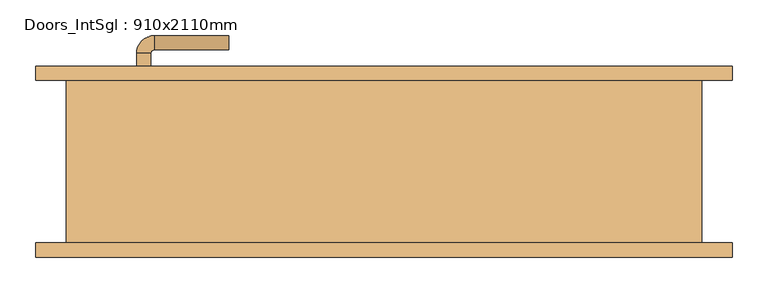
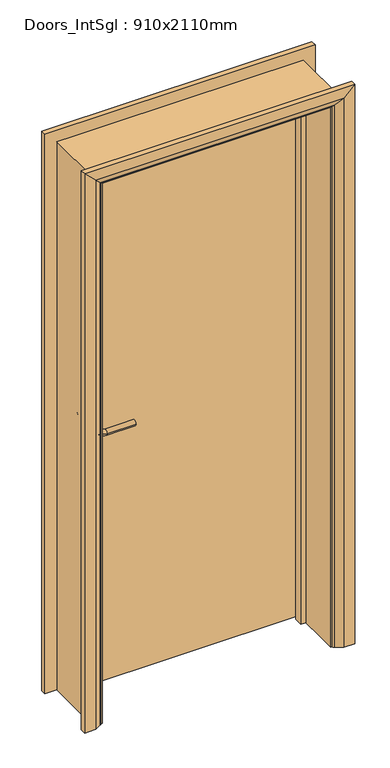
"""IFC4 building model written with IfcOpenShell, lengths in millimetres: door geometry, Doors_IntSgl : 910x2110mm."""

from ifc_helpers import new_model, si_unit, point, frame, frame_2d, origin, place, context, project, spatial, polyline, circle_curve, ellipse_curve, trimmed, segment, composite_curve, outline, extrude, faceted_brep, source, transform, mapped, element, save
from ifc_brep_helpers import plane_surface, cylinder_surface, revolved_surface, advanced_brep


def doors_intsgl_910x2110mm_6866c2a0(model_context):
    return source(origin(), model_context, "Body", "SolidModel", [
        advanced_brep(
        [(-348.0, 68.3, 1000.0), (-328.0, 68.3, 1000.0), (-328.0, 38.3, 1000.0), (-348.0, 38.3, 1000.0), (-323.0, 33.3, 1000.0), (-323.0, 13.3, 1000.0), (-218.0, 13.3, 1000.0), (-218.0, 33.3, 1000.0)],
        [
            (0, 1, circle_curve(frame((-338.0, 68.3, 1000.0), z_axis=(0.0, 1.0, 0.0), x_axis=(1.0, 0.0, 0.0)), 10.0)),
            (1, 0, circle_curve(frame((-338.0, 68.3, 1000.0), z_axis=(0.0, 1.0, 0.0), x_axis=(1.0, 0.0, 0.0)), 10.0)),
            (1, 2),
            (2, 3, circle_curve(frame((-338.0, 38.3, 1000.0), z_axis=(0.0, 1.0, 0.0), x_axis=(1.0, 0.0, 0.0)), 10.0)),
            (3, 0),
            (3, 2, circle_curve(frame((-338.0, 38.3, 1000.0), z_axis=(0.0, 1.0, 0.0), x_axis=(1.0, 0.0, 0.0)), 10.0)),
            (4, 5, circle_curve(frame((-323.0, 23.3, 1000.0), z_axis=(-1.0, 0.0, 0.0), x_axis=(0.0, 1.0, 0.0)), 10.0)),
            (5, 3, circle_curve(frame((-323.0, 38.3, 1000.0), z_axis=(0.0, 0.0, -1.0), x_axis=(-1.0, 0.0, 0.0)), 25.0)),
            (2, 4, circle_curve(frame((-323.0, 38.3, 1000.0), z_axis=(0.0, 0.0, 1.0), x_axis=(-1.0, 0.0, 0.0)), 5.0)),
            (5, 4, circle_curve(frame((-323.0, 23.3, 1000.0), z_axis=(-1.0, 0.0, 0.0), x_axis=(0.0, 1.0, 0.0)), 10.0)),
            (6, 7, circle_curve(frame((-218.0, 23.3, 1000.0), z_axis=(1.0, 0.0, 0.0), x_axis=(0.0, 1.0, 0.0)), 10.0)),
            (7, 6, circle_curve(frame((-218.0, 23.3, 1000.0), z_axis=(1.0, 0.0, 0.0), x_axis=(0.0, 1.0, 0.0)), 10.0)),
            (4, 7),
            (6, 5),
        ],
        [
            plane_surface(frame((-338.0, 68.3, 1000.0), z_axis=(0.0, 1.0, 0.0), x_axis=(0.0, 0.0, 1.0))),
            cylinder_surface(frame((-338.0, 68.3, 1000.0), z_axis=(0.0, 1.0, 0.0), x_axis=(1.0, 0.0, 0.0)), 10.0),
            revolved_surface(trimmed(ellipse_curve(frame((-338.0, 38.3, 1000.0), z_axis=(0.0, -1.0, 0.0), x_axis=(1.0, 0.0, 0.0)), 10.0, 10.0), [point((-348.0, 38.3, 1000.0))], [point((-328.0, 38.3, 1000.0))], True, "CARTESIAN"), (-323.0, 38.3, 1000.0), (0.0, 0.0, -1.0)),
            revolved_surface(trimmed(ellipse_curve(frame((-338.0, 38.3, 1000.0), z_axis=(0.0, -1.0, 0.0), x_axis=(1.0, 0.0, 0.0)), 10.0, 10.0), [point((-328.0, 38.3, 1000.0))], [point((-348.0, 38.3, 1000.0))], True, "CARTESIAN"), (-323.0, 38.3, 1000.0), (0.0, 0.0, -1.0)),
            plane_surface(frame((-218.0, 23.3, 1000.0), z_axis=(1.0, 0.0, 0.0), x_axis=(0.0, 0.0, 1.0))),
            cylinder_surface(frame((-323.0, 23.3, 1000.0), z_axis=(-1.0, 0.0, 0.0), x_axis=(0.0, 1.0, 0.0)), 10.0),
        ],
        [
            (0, [[1, 2]]),
            (1, [[3, 4, 5, -2]]),
            (1, [[-5, 6, -3, -1]]),
            (2, [[7, 8, -4, 9]]),
            (3, [[10, -9, -6, -8]]),
            (4, [[11, 12]]),
            (5, [[13, -11, 14, -7]]),
            (5, [[-14, -12, -13, -10]]),
        ],
    ),
        extrude(outline(composite_curve([segment(trimmed(circle_curve(frame_2d((1000.0, -340.5)), 30.0), [point((1000.0, -370.5))], [point((1000.0, -310.5))], False, "CARTESIAN"), True, "CONTINUOUS"), segment(trimmed(circle_curve(frame_2d((1000.0, -340.5)), 30.0), [point((1000.0, -310.5))], [point((1000.0, -370.5))], False, "CARTESIAN"), True, "CONTINUOUS")], self_intersect=False)), frame((0.0, 68.3, 0.0), z_axis=(0.0, 1.0, 0.0), x_axis=(0.0, 0.0, 1.0)), (0.0, 0.0, 1.0), 8.0),
        advanced_brep(
        [(-348.0, 122.3, 1000.0), (-328.0, 122.3, 1000.0), (-348.0, 152.3, 1000.0), (-328.0, 152.3, 1000.0), (-323.0, 157.3, 1000.0), (-323.0, 177.3, 1000.0), (-218.0, 177.3, 1000.0), (-218.0, 157.3, 1000.0)],
        [
            (0, 1, circle_curve(frame((-338.0, 122.3, 1000.0), z_axis=(0.0, -1.0, 0.0), x_axis=(1.0, 0.0, 0.0)), 10.0)),
            (1, 0, circle_curve(frame((-338.0, 122.3, 1000.0), z_axis=(0.0, -1.0, 0.0), x_axis=(1.0, 0.0, 0.0)), 10.0)),
            (0, 2),
            (2, 3, circle_curve(frame((-338.0, 152.3, 1000.0), z_axis=(0.0, -1.0, 0.0), x_axis=(1.0, 0.0, 0.0)), 10.0)),
            (3, 1),
            (3, 2, circle_curve(frame((-338.0, 152.3, 1000.0), z_axis=(0.0, -1.0, 0.0), x_axis=(1.0, 0.0, 0.0)), 10.0)),
            (4, 3, circle_curve(frame((-323.0, 152.3, 1000.0), z_axis=(0.0, 0.0, 1.0), x_axis=(-1.0, 0.0, 0.0)), 5.0)),
            (2, 5, circle_curve(frame((-323.0, 152.3, 1000.0), z_axis=(0.0, 0.0, -1.0), x_axis=(-1.0, 0.0, 0.0)), 25.0)),
            (5, 4, circle_curve(frame((-323.0, 167.3, 1000.0), z_axis=(-1.0, 0.0, 0.0), x_axis=(0.0, -1.0, 0.0)), 10.0)),
            (4, 5, circle_curve(frame((-323.0, 167.3, 1000.0), z_axis=(-1.0, 0.0, 0.0), x_axis=(0.0, -1.0, 0.0)), 10.0)),
            (6, 7, circle_curve(frame((-218.0, 167.3, 1000.0), z_axis=(1.0, 0.0, 0.0), x_axis=(0.0, -1.0, 0.0)), 10.0)),
            (7, 6, circle_curve(frame((-218.0, 167.3, 1000.0), z_axis=(1.0, 0.0, 0.0), x_axis=(0.0, -1.0, 0.0)), 10.0)),
            (5, 6),
            (7, 4),
        ],
        [
            plane_surface(frame((-338.0, 122.3, 1000.0), z_axis=(0.0, -1.0, 0.0), x_axis=(0.0, 0.0, 1.0))),
            cylinder_surface(frame((-338.0, 122.3, 1000.0), z_axis=(0.0, -1.0, 0.0), x_axis=(1.0, 0.0, 0.0)), 10.0),
            revolved_surface(trimmed(ellipse_curve(frame((-338.0, 152.3, 1000.0), z_axis=(0.0, -1.0, 0.0), x_axis=(1.0, 0.0, 0.0)), 10.0, 10.0), [point((-348.0, 152.3, 1000.0))], [point((-328.0, 152.3, 1000.0))], True, "CARTESIAN"), (-323.0, 152.3, 1000.0), (0.0, 0.0, -1.0)),
            revolved_surface(trimmed(ellipse_curve(frame((-338.0, 152.3, 1000.0), z_axis=(0.0, -1.0, 0.0), x_axis=(1.0, 0.0, 0.0)), 10.0, 10.0), [point((-328.0, 152.3, 1000.0))], [point((-348.0, 152.3, 1000.0))], True, "CARTESIAN"), (-323.0, 152.3, 1000.0), (0.0, 0.0, -1.0)),
            plane_surface(frame((-218.0, 167.3, 1000.0), z_axis=(1.0, 0.0, 0.0), x_axis=(0.0, 0.0, 1.0))),
            cylinder_surface(frame((-323.0, 167.3, 1000.0), z_axis=(-1.0, 0.0, 0.0), x_axis=(0.0, -1.0, 0.0)), 10.0),
        ],
        [
            (0, [[1, 2]]),
            (1, [[-1, 3, 4, 5]]),
            (1, [[-2, -5, 6, -3]]),
            (2, [[7, -4, 8, 9]]),
            (3, [[-8, -6, -7, 10]]),
            (4, [[11, 12]]),
            (5, [[-9, 13, -12, 14]]),
            (5, [[-10, -14, -11, -13]]),
        ],
    ),
        extrude(outline(composite_curve([segment(trimmed(circle_curve(frame_2d((1000.0, -340.5)), 30.0), [point((1000.0, -370.5))], [point((1000.0, -310.5))], False, "CARTESIAN"), True, "CONTINUOUS"), segment(trimmed(circle_curve(frame_2d((1000.0, -340.5)), 30.0), [point((1000.0, -310.5))], [point((1000.0, -370.5))], False, "CARTESIAN"), True, "CONTINUOUS")], self_intersect=False)), frame((0.0, 114.3, 0.0), z_axis=(0.0, 1.0, 0.0), x_axis=(0.0, 0.0, 1.0)), (0.0, 0.0, 1.0), 8.0),
        extrude(outline(polyline([(413.0, 76.3), (-413.0, 76.3), (-413.0, 114.3), (413.0, 114.3), (413.0, 76.3)])), frame((0.0, 0.0, 8.0), z_axis=(0.0, 0.0, 1.0), x_axis=(1.0, 0.0, 0.0)), (0.0, 0.0, 1.0), 2060.0),
        advanced_brep(
        [(490.0, 134.3, 0.0), (490.0, 114.3, 0.0), (420.0, 114.3, 0.0), (424.0, 120.3, 0.0), (450.0, 134.3, 0.0), (490.0, 134.3, 2145.0), (490.0, 114.3, 2145.0), (-490.0, 114.3, 2145.0), (-490.0, 114.3, 0.0), (-420.0, 114.3, 0.0), (-420.0, 114.3, 2075.0), (420.0, 114.3, 2075.0), (424.0, 120.3, 2079.0), (450.0, 134.3, 2105.0), (-450.0, 134.3, 2105.0), (-450.0, 134.3, 0.0), (-490.0, 134.3, 0.0), (-490.0, 134.3, 2145.0), (-424.0, 120.3, 2079.0), (-424.0, 120.3, 0.0)],
        [
            (0, 1),
            (1, 2),
            (2, 3, circle_curve(frame((428.0, 113.3, 0.0), z_axis=(0.0, 0.0, -1.0), x_axis=(1.0, 0.0, 0.0)), 8.0622577)),
            (3, 4),
            (4, 0),
            (0, 5),
            (5, 6),
            (6, 1),
            (6, 7),
            (7, 8),
            (8, 9),
            (9, 10),
            (10, 11),
            (11, 2),
            (11, 12, ellipse_curve(frame((428.0, 113.3, 2083.0), z_axis=(0.7071067811865475, 0.0, -0.7071067811865475), x_axis=(-0.7071067811865474, 0.0, -0.7071067811865476)), 11.4017543, 8.0622577)),
            (12, 3),
            (12, 13),
            (13, 4),
            (13, 14),
            (14, 15),
            (15, 16),
            (16, 17),
            (17, 5),
            (17, 7),
            (10, 18, ellipse_curve(frame((-428.0, 113.3, 2083.0), z_axis=(0.7071067811865475, 0.0, 0.7071067811865475), x_axis=(0.7071067811865476, 0.0, -0.7071067811865474)), 11.4017543, 8.0622577)),
            (18, 12),
            (18, 14),
            (15, 19),
            (19, 9, circle_curve(frame((-428.0, 113.3, 0.0), z_axis=(0.0, 0.0, -1.0), x_axis=(-1.0, 0.0, 0.0)), 8.0622577)),
            (8, 16),
            (19, 18),
        ],
        [
            plane_surface(frame((420.0, 114.3, 0.0), z_axis=(0.0, 0.0, -1.0), x_axis=(0.0, -1.0, 0.0))),
            plane_surface(frame((490.0, 134.3, 0.0), z_axis=(1.0, 0.0, 0.0), x_axis=(0.0, 0.0, 1.0))),
            plane_surface(frame((490.0, 114.3, 0.0), z_axis=(0.0, -1.0, 0.0), x_axis=(0.0, 0.0, 1.0))),
            cylinder_surface(frame((428.0, 113.3, 0.0), z_axis=(0.0, 0.0, -1.0), x_axis=(1.0, 0.0, 0.0)), 8.0622577),
            plane_surface(frame((424.0, 120.3, 0.0), z_axis=(-0.4740998230350126, 0.880471099922178, 0.0), x_axis=(0.0, 0.0, 1.0))),
            plane_surface(frame((450.0, 134.3, 0.0), z_axis=(0.0, 1.0, 0.0), x_axis=(0.0, 0.0, 1.0))),
            plane_surface(frame((490.0, 134.3, 2145.0), z_axis=(0.0, 0.0, 1.0), x_axis=(-1.0, 0.0, 0.0))),
            cylinder_surface(frame((420.0, 113.3, 2083.0), z_axis=(1.0, 0.0, 0.0), x_axis=(0.0, 0.0, 1.0)), 8.0622577),
            plane_surface(frame((424.0, 120.3, 2079.0), z_axis=(0.0, 0.8804710999221764, -0.4740998230350154), x_axis=(-1.0, 0.0, 0.0))),
            plane_surface(frame((-420.0, 114.3, 0.0), z_axis=(0.0, 0.0, -1.0), x_axis=(0.0, -1.0, 0.0))),
            plane_surface(frame((-490.0, 134.3, 2145.0), z_axis=(-1.0, 0.0, 0.0), x_axis=(0.0, 0.0, -1.0))),
            cylinder_surface(frame((-428.0, 113.3, 2075.0), z_axis=(0.0, 0.0, 1.0), x_axis=(-1.0, 0.0, 0.0)), 8.0622577),
            plane_surface(frame((-424.0, 120.3, 2079.0), z_axis=(0.47409982303501824, 0.8804710999221749, 0.0), x_axis=(0.0, 0.0, -1.0))),
        ],
        [
            (0, [[1, 2, 3, 4, 5]]),
            (1, [[-1, 6, 7, 8]]),
            (2, [[-2, -8, 9, 10, 11, 12, 13, 14]]),
            (3, [[-3, -14, 15, 16]]),
            (4, [[-4, -16, 17, 18]]),
            (5, [[-5, -18, 19, 20, 21, 22, 23, -6]]),
            (6, [[-7, -23, 24, -9]]),
            (7, [[-15, -13, 25, 26]]),
            (8, [[-17, -26, 27, -19]]),
            (9, [[-21, 28, 29, -11, 30]]),
            (10, [[-24, -22, -30, -10]]),
            (11, [[-25, -12, -29, 31]]),
            (12, [[-27, -31, -28, -20]]),
        ],
    ),
        extrude(outline(polyline([(0.0, -415.0), (0.0, -396.0), (2051.0, -396.0), (2051.0, 396.0), (0.0, 396.0), (0.0, 415.0), (2070.0, 415.0), (2070.0, -415.0), (0.0, -415.0)])), frame((0.0, 42.3, 0.0), z_axis=(0.0, 1.0, 0.0), x_axis=(0.0, 0.0, 1.0)), (0.0, 0.0, 1.0), 32.0),
        advanced_brep(
        [(-490.0, -134.3, 0.0), (-490.0, -114.3, 0.0), (-420.0, -114.3, 0.0), (-424.0, -120.3, 0.0), (-450.0, -134.3, 0.0), (-490.0, -134.3, 2145.0), (-490.0, -114.3, 2145.0), (-420.0, -114.3, 2075.0), (-424.0, -120.3, 2079.0), (-450.0, -134.3, 2105.0), (490.0, -134.3, 2145.0), (490.0, -114.3, 2145.0), (420.0, -114.3, 2075.0), (424.0, -120.3, 2079.0), (450.0, -134.3, 2105.0), (490.0, -134.3, 0.0), (450.0, -134.3, 0.0), (424.0, -120.3, 0.0), (420.0, -114.3, 0.0), (490.0, -114.3, 0.0)],
        [
            (0, 1),
            (1, 2),
            (2, 3, circle_curve(frame((-428.0, -113.3, 0.0), z_axis=(0.0, 0.0, -1.0), x_axis=(-1.0, 0.0, 0.0)), 8.0622577)),
            (3, 4),
            (4, 0),
            (0, 5),
            (5, 6),
            (6, 1),
            (6, 7),
            (7, 2),
            (7, 8, ellipse_curve(frame((-428.0, -113.3, 2083.0), z_axis=(-0.7071067811865475, 0.0, -0.7071067811865475), x_axis=(0.7071067811865474, 0.0, -0.7071067811865476)), 11.4017543, 8.0622577)),
            (8, 3),
            (8, 9),
            (9, 4),
            (9, 5),
            (5, 10),
            (10, 11),
            (11, 6),
            (11, 12),
            (12, 7),
            (12, 13, ellipse_curve(frame((428.0, -113.3, 2083.0), z_axis=(-0.7071067811865475, 0.0, 0.7071067811865475), x_axis=(-0.7071067811865476, 0.0, -0.7071067811865474)), 11.4017543, 8.0622577)),
            (13, 8),
            (13, 14),
            (14, 9),
            (14, 10),
            (15, 16),
            (16, 17),
            (17, 18, circle_curve(frame((428.0, -113.3, 0.0), z_axis=(0.0, 0.0, -1.0), x_axis=(1.0, 0.0, 0.0)), 8.0622577)),
            (18, 19),
            (19, 15),
            (10, 15),
            (19, 11),
            (18, 12),
            (17, 13),
            (16, 14),
        ],
        [
            plane_surface(frame((-420.0, -187.1010989, 0.0), z_axis=(0.0, 0.0, -1.0), x_axis=(1.0, 0.0, 0.0))),
            plane_surface(frame((-490.0, -134.3, 0.0), z_axis=(-1.0, 0.0, 0.0), x_axis=(0.0, 0.0, 1.0))),
            plane_surface(frame((-490.0, -114.3, 0.0), z_axis=(0.0, 1.0, 0.0), x_axis=(0.0, 0.0, 1.0))),
            cylinder_surface(frame((-428.0, -113.3, 0.0), z_axis=(0.0, 0.0, -1.0), x_axis=(-1.0, 0.0, 0.0)), 8.0622577),
            plane_surface(frame((-424.0, -120.3, 0.0), z_axis=(0.4740998230350183, -0.8804710999221749, 0.0), x_axis=(0.0, 0.0, 1.0))),
            plane_surface(frame((-450.0, -134.3, 0.0), z_axis=(0.0, -1.0, 0.0), x_axis=(0.0, 0.0, 1.0))),
            plane_surface(frame((-490.0, -134.3, 2145.0), z_axis=(0.0, 0.0, 1.0), x_axis=(1.0, 0.0, 0.0))),
            plane_surface(frame((-490.0, -114.3, 2145.0), z_axis=(0.0, 1.0, 0.0), x_axis=(1.0, 0.0, 0.0))),
            cylinder_surface(frame((-420.0, -113.3, 2083.0), z_axis=(-1.0, 0.0, 0.0), x_axis=(0.0, 0.0, 1.0)), 8.0622577),
            plane_surface(frame((-424.0, -120.3, 2079.0), z_axis=(0.0, -0.8804710999221749, -0.4740998230350183), x_axis=(1.0, 0.0, 0.0))),
            plane_surface(frame((-450.0, -134.3, 2105.0), z_axis=(0.0, -1.0, 0.0), x_axis=(1.0, 0.0, 0.0))),
            plane_surface(frame((420.0, -187.1010989, 0.0), z_axis=(0.0, 0.0, -1.0), x_axis=(-1.0, 0.0, 0.0))),
            plane_surface(frame((490.0, -134.3, 2145.0), z_axis=(1.0, 0.0, 0.0), x_axis=(0.0, 0.0, -1.0))),
            plane_surface(frame((490.0, -114.3, 2145.0), z_axis=(0.0, 1.0, 0.0), x_axis=(0.0, 0.0, -1.0))),
            cylinder_surface(frame((428.0, -113.3, 2075.0), z_axis=(0.0, 0.0, 1.0), x_axis=(1.0, 0.0, 0.0)), 8.0622577),
            plane_surface(frame((424.0, -120.3, 2079.0), z_axis=(-0.4740998230350183, -0.8804710999221749, 0.0), x_axis=(0.0, 0.0, -1.0))),
            plane_surface(frame((450.0, -134.3, 2105.0), z_axis=(0.0, -1.0, 0.0), x_axis=(0.0, 0.0, -1.0))),
        ],
        [
            (0, [[1, 2, 3, 4, 5]]),
            (1, [[-1, 6, 7, 8]]),
            (2, [[-2, -8, 9, 10]]),
            (3, [[-3, -10, 11, 12]]),
            (4, [[-4, -12, 13, 14]]),
            (5, [[-5, -14, 15, -6]]),
            (6, [[-7, 16, 17, 18]]),
            (7, [[-9, -18, 19, 20]]),
            (8, [[-11, -20, 21, 22]]),
            (9, [[-13, -22, 23, 24]]),
            (10, [[-15, -24, 25, -16]]),
            (11, [[26, 27, 28, 29, 30]]),
            (12, [[-17, 31, -30, 32]]),
            (13, [[-19, -32, -29, 33]]),
            (14, [[-21, -33, -28, 34]]),
            (15, [[-23, -34, -27, 35]]),
            (16, [[-25, -35, -26, -31]]),
        ],
    ),
        faceted_brep([(-415.0, 114.3, 0.0), (-415.0, -114.3, 0.0), (-447.0, -114.3, 0.0), (-447.0, 114.3, 0.0), (-415.0, 114.3, 2070.0), (-415.0, -114.3, 2070.0), (-447.0, -114.3, 2102.0), (-447.0, 114.3, 2102.0), (415.0, 114.3, 2070.0), (415.0, -114.3, 2070.0), (447.0, -114.3, 2102.0), (447.0, 114.3, 2102.0), (415.0, 114.3, 0.0), (447.0, 114.3, 0.0), (447.0, -114.3, 0.0), (415.0, -114.3, 0.0)], [[[0, 1, 2, 3]], [[1, 0, 4, 5]], [[2, 1, 5, 6]], [[3, 2, 6, 7]], [[0, 3, 7, 4]], [[5, 4, 8, 9]], [[6, 5, 9, 10]], [[7, 6, 10, 11]], [[4, 7, 11, 8]], [[12, 13, 14, 15]], [[9, 8, 12, 15]], [[10, 9, 15, 14]], [[11, 10, 14, 13]], [[8, 11, 13, 12]]]),
    ])


if __name__ == "__main__":
    model = new_model("IFC4")
    model_context = context("Model", 3, world=origin())
    ifc_project = project(units=[si_unit("LENGTHUNIT", "METRE", prefix="MILLI")], contexts=[model_context])
    site = spatial("IfcSite", under=ifc_project)
    building = spatial("IfcBuilding", under=site)
    placement = place(None, origin())
    doors_intsgl_910x2110mm_shape = doors_intsgl_910x2110mm_6866c2a0(model_context)
    element("IfcDoor", 1, ObjectType="Doors_IntSgl : 910x2110mm", at=placement, inside=building, context=model_context, shape_type="MappedRepresentation", body=[
        mapped(doors_intsgl_910x2110mm_shape, transform((0.0, 0.0, 0.0), x_axis=(1.0, 0.0, 0.0), y_axis=(0.0, 1.0, 0.0), z_axis=(0.0, 0.0, 1.0))),
    ])
    save(model, "model.ifc")

# Revit data of these elements
# Type "Doors_IntSgl : 910x2110mm"
#   Construction Type Id = "MDOOR"
#   Type Mark = "41"
#   Type Comments = "Internal Single"
#   Operation = "SingleSwingRight"
#   Manufacturer = "Revit"
#   Keynote = "L20"
#   Description = "Internal Single Door"
#   Analytic Construction = "Metal"
#   UnderCut = 0' - 0.31496"
#   Tolerance = 0' - 0.07874"
#   Thickness = 0' - 1.49606"
#   Thermal Resistance (R) = 0.270117 (m²·K)/W
#   Structural Tolerance = 0' - 0.31496"
#   StopDepth = 0' - 1.25984"
#   Stop Thickness = 0' - 0.74803"
#   Rough Width = 2' - 11.82677"
#   Rough Height = 6' - 11.07087"
#   Height to Top Lock Rail = 3' - 3.37008"
#   Heat Transfer Coefficient (U) = 3.7021 W/(m²·K)
#   Handle Z Distance = 3' - 3.37008"
#   Handle X Distance = 0' - 2.95276"
#   Frame Thickness = 0' - 1.25984"
#   Door Panel Width = 2' - 8.51969"
#   Door Panel Thickness = 0' - 1.49606"
#   Door Panel Offset = 0' - 0"
#   Height = 6' - 11.07087"
#   Width = 2' - 11.82677"
#   Door Panel Height = 6' - 9.10236"
#   Architrave Setback = 0' - 0.19685"
#   Define Thermal Properties by = 1
#   Vis - Ironmongery = yes
#   Material Ironmongery = Door - Handle
#   Material Frame = Door - Frame/Mullion (1)
#   Material Door = Door - Panel
#   Material Architrave = Door - Architrave
#   Visual Light Transmittance = 0
#   Solar Heat Gain Coefficient = 0
#   Function = (empty or 0)
#   Wall Closure = (empty or 0)
# Element 1 (IfcDoor, "Doors_IntSgl : 910x2110mm")
#   Materials on its faces: "Door - Architrave", "Door - Handle", "Door - Frame/Mullion (1)", "Door - Panel"
# Materials
#   "Door - Handle": colour RGB 0 0 0, transparency 0, Keynote = "P21", Cost = 0
#   "Door - Frame/Mullion (1)": class "Wood", colour RGB 212 179 113, transparency 0, Keynote = "L20", Cost = 0
#   "Door - Panel": class "Wood", colour RGB 210 159 95, transparency 0, Keynote = "L20", Cost = 0
#   "Door - Architrave": class "Wood", colour RGB 154 90 5, transparency 0, Keynote = "P20", Cost = 0
